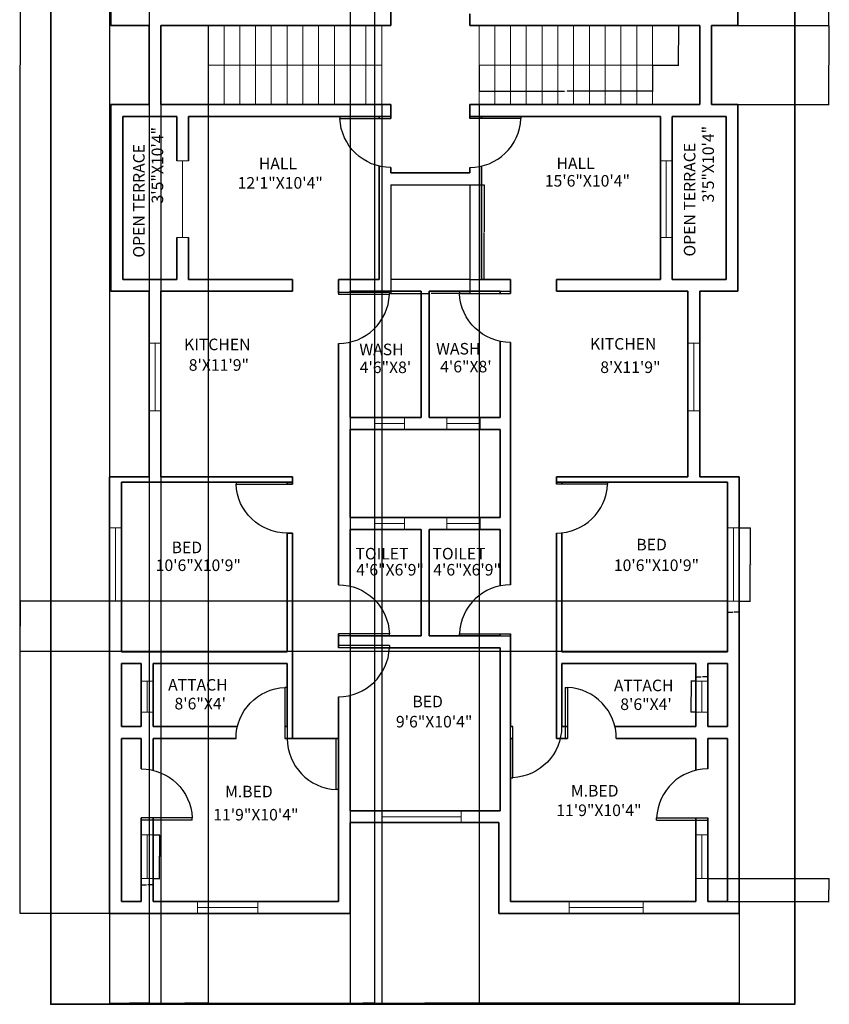
# Model space of a CAD drawing. Units: feet. Extents: x 100807 to 101423, y 154875 to 156331.
# Tile 1 of 8: x 100807 to 101423, y 154875 to 155624. Entities that reach past the tile are written whole.
import ezdxf

# ---------------------------------------------------------------- set-up
doc = ezdxf.new("R2010")
doc.units = ezdxf.units.FT
for name, color, linetype, lineweight in [('A-ANNO-DIMS', 2, 'Continuous', 18), ('A-ANNO-TTLB', 7, 'Continuous', 35), ('A-AREA-IDEN', 7, 'Continuous', 25), ('A-DOOR', 4, 'Continuous', 25), ('A-EQPM-ELEV', 8, 'Continuous', 25), ('A-FLOR-STRS', 3, 'Continuous', 18), ('A-GLAZ', 4, 'Continuous', 18), ('A-WALL', 7, 'Continuous', 35)]:
    doc.layers.add(name, color=color, linetype=linetype, lineweight=lineweight)
doc.styles.get("Standard").update_dxf_attribs({"font": 'arial.ttf'})
doc.dimstyles.get("Standard").update_dxf_attribs({"dimtxt": 0.18, "dimasz": 0.18, "dimexe": 0.18, "dimexo": 0.0625, "dimgap": 0.09, "dimtad": 0, "dimtih": 1, "dimtoh": 1, "dimdec": 4, "dimzin": 0, "dimdsep": 46, "dimtxsty": 'Standard', "dimcen": 0.09, "dimadec": 0, "dimazin": 0, "dimtfac": 1, "dimtdec": 4, "dimtofl": 0, "dimtmove": 0, "dimatfit": 3, "dimfxl": 1, "dimtolj": 1, "dimtzin": 0, "dimarcsym": 0})

# ---------------------------------------------------------------- blocks, each defined once
blk = doc.blocks.new('DR-36')
for p, q in [((0, 36), (0, 0)), ((0, 36), (1.5, 36)), ((1.5, 36), (1.5, 0)), ((0, 0), (1.5, 0))]:
    blk.add_line(p, q)
blk.add_arc((0, 0), 36, 0, 87.61406)
blk = doc.blocks.new('VENT-COURT-A')
for p, q in [((0, 9), (0, 0)), ((22.83, 9), (22.83, 0)), ((22.83, 4.5), (0, 4.5))]:
    blk.add_line(p, q)
blk = doc.blocks.new('WIN-BATH-SIDE')
for p, q in [((0, 23.54), (9, 23.54)), ((4.5, 23.54), (4.5, 0)), ((0, 0), (9, 0))]:
    blk.add_line(p, q)
blk = doc.blocks.new('VENT-COURT-B')
for p, q in [((0, 9), (0, 0)), ((25.42, 9), (25.42, 0)), ((25.42, 4.5), (0, 4.5))]:
    blk.add_line(p, q)
blk = doc.blocks.new('WIN-MBED-SIDE')
for p, q in [((0, 33.08), (9, 33.08)), ((4.5, 33.08), (4.5, 0)), ((0, 0), (9, 0))]:
    blk.add_line(p, q)
blk = doc.blocks.new('WIN-KITCHEN')
for p, q in [((0, 51.58), (9, 51.58)), ((4.5, 51.58), (4.5, 0)), ((0, 0), (9, 0))]:
    blk.add_line(p, q)
blk = doc.blocks.new('WIN-BED-SIDE')
for p, q in [((0, 55.85), (9, 55.85)), ((4.5, 55.85), (4.5, 0)), ((0, 0), (9, 0))]:
    blk.add_line(p, q)
blk = doc.blocks.new('WIN-TERRACE')
for p, q in [((0, 58.29), (9, 58.29)), ((4.5, 58.29), (4.5, 0)), ((0, 0), (9, 0))]:
    blk.add_line(p, q)
blk = doc.blocks.new('WIN-BED-END')
for p, q in [((0, 9), (0, 0)), ((60.14, 9), (60.14, 0)), ((0, 4.5), (60.14, 4.5))]:
    blk.add_line(p, q)
blk = doc.blocks.new('STAIR-FLIGHT-12')
for p, q in [((0, 30), (0, 0)), ((12, 30), (12, 0)), ((24, 30), (24, 0)), ((36, 30), (36, 0)), ((48, 30), (48, 0)), ((60, 30), (60, 0)), ((72, 30), (72, 0)), ((84, 30), (84, 0)), ((96, 30), (96, 0)), ((108, 30), (108, 0)), ((120, 30), (120, 0)), ((132, 30), (132, 0))]:
    blk.add_line(p, q)
blk = doc.blocks.new('LIFT-OUTLINE')
for p, q in [((0, 72), (0, 0)), ((0, 72), (60, 72)), ((60, 72), (60, 0)), ((60, 72), (60, 0)), ((60, 0), (0, 0))]:
    blk.add_line(p, q)
blk = doc.blocks.new('*D18')
at = {"layer": 'A-ANNO-DIMS', "color": 0, "lineweight": -2, "transparency": 16777216}
for p, q in [((101321.09, 155121.03), (101317.44, 155121.03)), ((101317.62, 155120.85), (101317.62, 155109.44)), ((101317.62, 155097.66), (101317.62, 155109.08)), ((101321.09, 155097.48), (101317.44, 155097.48))]:
    blk.add_line(p, q, dxfattribs=at)
at = {"layer": 'A-ANNO-DIMS', "color": 0, "transparency": 16777216}
for points in [[(101317.59, 155120.85), (101317.65, 155120.85), (101317.62, 155121.03)], [(101317.59, 155097.66), (101317.65, 155097.66), (101317.62, 155097.48)]]:
    blk.add_solid(points, dxfattribs=at)
at = {"layer": 'Defpoints', "color": 0, "transparency": 16777216}
for p in [(101321.16, 155121.03), (101317.62, 155097.48), (101321.16, 155097.48)]:
    blk.add_point(p, dxfattribs=at)
at = {"layer": 'A-ANNO-DIMS', "color": 0, "transparency": 16777216, "insert": (101317.62, 155109.26), "char_height": 0.18, "attachment_point": 5}
blk.add_mtext('\\A1;BATH WIN. 24 TYP.', dxfattribs=at)
blk = doc.blocks.new('*D19')
at = {"layer": 'A-ANNO-DIMS', "color": 0, "lineweight": -2, "transparency": 16777216}
for p, q in [((101321.16, 155121.09), (101321.16, 155124.74)), ((101321.34, 155124.56), (101325.2, 155124.56)), ((101329.98, 155124.56), (101326.11, 155124.56)), ((101330.16, 155121.09), (101330.16, 155124.74))]:
    blk.add_line(p, q, dxfattribs=at)
at = {"layer": 'A-ANNO-DIMS', "color": 0, "transparency": 16777216}
for points in [[(101321.34, 155124.59), (101321.34, 155124.53), (101321.16, 155124.56)], [(101329.98, 155124.59), (101329.98, 155124.53), (101330.16, 155124.56)]]:
    blk.add_solid(points, dxfattribs=at)
at = {"layer": 'Defpoints', "color": 0, "transparency": 16777216}
for p in [(101321.16, 155124.56), (101321.16, 155121.03), (101330.16, 155121.03)]:
    blk.add_point(p, dxfattribs=at)
at = {"layer": 'A-ANNO-DIMS', "color": 0, "transparency": 16777216, "insert": (101325.66, 155124.56), "char_height": 0.18, "attachment_point": 5}
blk.add_mtext('\\A1;9 TYP.', dxfattribs=at)
blk = doc.blocks.new('*D20')
at = {"layer": 'A-ANNO-DIMS', "color": 0, "lineweight": -2, "transparency": 16777216}
for p, q in [((100908.22, 155004.3), (100913.3, 155004.3)), ((100913.12, 155004.12), (100913.12, 154987.95)), ((100913.12, 154971.41), (100913.12, 154987.58)), ((100908.22, 154971.23), (100913.3, 154971.23))]:
    blk.add_line(p, q, dxfattribs=at)
at = {"layer": 'A-ANNO-DIMS', "color": 0, "transparency": 16777216}
for points in [[(100913.09, 155004.12), (100913.15, 155004.12), (100913.12, 155004.3)], [(100913.09, 154971.41), (100913.15, 154971.41), (100913.12, 154971.23)]]:
    blk.add_solid(points, dxfattribs=at)
at = {"layer": 'Defpoints', "color": 0, "transparency": 16777216}
for p in [(100908.16, 155004.3), (100908.16, 154971.23), (100913.12, 154971.23)]:
    blk.add_point(p, dxfattribs=at)
at = {"layer": 'A-ANNO-DIMS', "color": 0, "transparency": 16777216, "insert": (100913.12, 154987.76), "char_height": 0.18, "attachment_point": 5}
blk.add_mtext('\\A1;M.BED WIN. 33 TYP.', dxfattribs=at)
blk = doc.blocks.new('*D21')
at = {"layer": 'A-ANNO-DIMS', "color": 0, "lineweight": -2, "transparency": 16777216}
for p, q in [((100899.16, 154971.16), (100899.16, 154966.08)), ((100899.34, 154966.26), (100903.2, 154966.26)), ((100907.98, 154966.26), (100904.11, 154966.26)), ((100908.16, 154971.16), (100908.16, 154966.08))]:
    blk.add_line(p, q, dxfattribs=at)
at = {"layer": 'A-ANNO-DIMS', "color": 0, "transparency": 16777216}
for points in [[(100899.34, 154966.29), (100899.34, 154966.23), (100899.16, 154966.26)], [(100907.98, 154966.29), (100907.98, 154966.23), (100908.16, 154966.26)]]:
    blk.add_solid(points, dxfattribs=at)
at = {"layer": 'Defpoints', "color": 0, "transparency": 16777216}
for p in [(100899.16, 154971.23), (100899.16, 154966.26), (100908.16, 154971.23)]:
    blk.add_point(p, dxfattribs=at)
at = {"layer": 'A-ANNO-DIMS', "color": 0, "transparency": 16777216, "insert": (100903.66, 154966.26), "char_height": 0.18, "attachment_point": 5}
blk.add_mtext('\\A1;9 TYP.', dxfattribs=at)
blk = doc.blocks.new('*D24')
at = {"layer": 'A-ANNO-DIMS', "color": 0, "lineweight": -2, "transparency": 16777216}
for p, q in [((101354.22, 155237.85), (101362.71, 155237.85)), ((101362.53, 155237.67), (101362.53, 155210.11)), ((101362.53, 155182.19), (101362.53, 155209.75)), ((101354.22, 155182.01), (101362.71, 155182.01))]:
    blk.add_line(p, q, dxfattribs=at)
at = {"layer": 'A-ANNO-DIMS', "color": 0, "transparency": 16777216}
for points in [[(101362.5, 155237.67), (101362.56, 155237.67), (101362.53, 155237.85)], [(101362.5, 155182.19), (101362.56, 155182.19), (101362.53, 155182.01)]]:
    blk.add_solid(points, dxfattribs=at)
at = {"layer": 'Defpoints', "color": 0, "transparency": 16777216}
for p in [(101354.16, 155237.85), (101362.53, 155237.85), (101354.16, 155182.01)]:
    blk.add_point(p, dxfattribs=at)
at = {"layer": 'A-ANNO-DIMS', "color": 0, "transparency": 16777216, "insert": (101362.53, 155209.93), "char_height": 0.18, "attachment_point": 5}
blk.add_mtext('\\A1;BED WIN. 56 TYP.', dxfattribs=at)
blk = doc.blocks.new('*D25')
at = {"layer": 'A-ANNO-DIMS', "color": 0, "lineweight": -2, "transparency": 16777216}
for p, q in [((101345.16, 155181.94), (101345.16, 155173.45)), ((101354.16, 155181.94), (101354.16, 155173.45)), ((101345.34, 155173.63), (101349.2, 155173.63)), ((101353.98, 155173.63), (101350.11, 155173.63))]:
    blk.add_line(p, q, dxfattribs=at)
at = {"layer": 'A-ANNO-DIMS', "color": 0, "transparency": 16777216}
for points in [[(101345.34, 155173.66), (101345.34, 155173.6), (101345.16, 155173.63)], [(101353.98, 155173.66), (101353.98, 155173.6), (101354.16, 155173.63)]]:
    blk.add_solid(points, dxfattribs=at)
at = {"layer": 'Defpoints', "color": 0, "transparency": 16777216}
for p in [(101345.16, 155182.01), (101354.16, 155182.01), (101354.16, 155173.63)]:
    blk.add_point(p, dxfattribs=at)
at = {"layer": 'A-ANNO-DIMS', "color": 0, "transparency": 16777216, "insert": (101349.66, 155173.63), "char_height": 0.18, "attachment_point": 5}
blk.add_mtext('\\A1;9 TYP.', dxfattribs=at)
blk = doc.blocks.new('*D30')
at = {"layer": 'A-ANNO-DIMS', "color": 0, "lineweight": -2, "transparency": 16777216}
for p, q in [((101156.16, 155589.49), (101156.16, 155569.58)), ((101288.16, 155589.49), (101288.16, 155569.58)), ((101156.34, 155569.76), (101221.15, 155569.76)), ((101287.98, 155569.76), (101223.16, 155569.76))]:
    blk.add_line(p, q, dxfattribs=at)
at = {"layer": 'A-ANNO-DIMS', "color": 0, "transparency": 16777216}
for points in [[(101156.34, 155569.79), (101156.34, 155569.73), (101156.16, 155569.76)], [(101287.98, 155569.79), (101287.98, 155569.73), (101288.16, 155569.76)]]:
    blk.add_solid(points, dxfattribs=at)
at = {"layer": 'Defpoints', "color": 0, "transparency": 16777216}
for p in [(101156.16, 155589.56), (101288.16, 155589.56), (101288.16, 155569.76)]:
    blk.add_point(p, dxfattribs=at)
at = {"layer": 'A-ANNO-DIMS', "color": 0, "transparency": 16777216, "insert": (101222.16, 155569.76), "char_height": 0.18, "attachment_point": 5}
blk.add_mtext('\\A1;STAIR 132 TYP.', dxfattribs=at)
blk = doc.blocks.new('*D31')
at = {"layer": 'A-ANNO-DIMS', "color": 0, "lineweight": -2, "transparency": 16777216}
for p, q in [((101288.22, 155619.56), (101308.14, 155619.56)), ((101307.96, 155619.38), (101307.96, 155604.74)), ((101307.96, 155589.74), (101307.96, 155604.37)), ((101288.22, 155589.56), (101308.14, 155589.56))]:
    blk.add_line(p, q, dxfattribs=at)
at = {"layer": 'A-ANNO-DIMS', "color": 0, "transparency": 16777216}
for points in [[(101307.93, 155619.38), (101307.99, 155619.38), (101307.96, 155619.56)], [(101307.93, 155589.74), (101307.99, 155589.74), (101307.96, 155589.56)]]:
    blk.add_solid(points, dxfattribs=at)
at = {"layer": 'Defpoints', "color": 0, "transparency": 16777216}
for p in [(101288.16, 155619.56), (101307.96, 155619.56), (101288.16, 155589.56)]:
    blk.add_point(p, dxfattribs=at)
at = {"layer": 'A-ANNO-DIMS', "color": 0, "transparency": 16777216, "insert": (101307.96, 155604.56), "char_height": 0.18, "attachment_point": 5}
blk.add_mtext('\\A1;30 TYP.', dxfattribs=at)
blk = doc.blocks.new('*D32')
at = {"layer": 'A-ANNO-DIMS', "color": 0, "lineweight": -2, "transparency": 16777216}
for p, q in [((101149.22, 155498.58), (101160.14, 155498.58)), ((101159.96, 155498.4), (101159.96, 155462.76)), ((101159.96, 155426.76), (101159.96, 155462.4)), ((101149.22, 155426.58), (101160.14, 155426.58))]:
    blk.add_line(p, q, dxfattribs=at)
at = {"layer": 'A-ANNO-DIMS', "color": 0, "transparency": 16777216}
for points in [[(101159.93, 155498.4), (101159.99, 155498.4), (101159.96, 155498.58)], [(101159.93, 155426.76), (101159.99, 155426.76), (101159.96, 155426.58)]]:
    blk.add_solid(points, dxfattribs=at)
at = {"layer": 'Defpoints', "color": 0, "transparency": 16777216}
for p in [(101149.16, 155498.58), (101159.96, 155498.58), (101149.16, 155426.58)]:
    blk.add_point(p, dxfattribs=at)
at = {"layer": 'A-ANNO-DIMS', "color": 0, "transparency": 16777216, "insert": (101159.96, 155462.58), "char_height": 0.18, "attachment_point": 5}
blk.add_mtext('\\A1;LIFT 72 TYP.', dxfattribs=at)
blk = doc.blocks.new('*D33')
at = {"layer": 'A-ANNO-DIMS', "color": 0, "lineweight": -2, "transparency": 16777216}
for p, q in [((101089.16, 155426.52), (101089.16, 155415.6)), ((101149.16, 155426.52), (101149.16, 155415.6)), ((101089.34, 155415.78), (101118.63, 155415.78)), ((101148.98, 155415.78), (101119.69, 155415.78))]:
    blk.add_line(p, q, dxfattribs=at)
at = {"layer": 'A-ANNO-DIMS', "color": 0, "transparency": 16777216}
for points in [[(101089.34, 155415.81), (101089.34, 155415.75), (101089.16, 155415.78)], [(101148.98, 155415.81), (101148.98, 155415.75), (101149.16, 155415.78)]]:
    blk.add_solid(points, dxfattribs=at)
at = {"layer": 'Defpoints', "color": 0, "transparency": 16777216}
for p in [(101089.16, 155426.58), (101149.16, 155426.58), (101149.16, 155415.78)]:
    blk.add_point(p, dxfattribs=at)
at = {"layer": 'A-ANNO-DIMS', "color": 0, "transparency": 16777216, "insert": (101119.16, 155415.78), "char_height": 0.18, "attachment_point": 5}
blk.add_mtext('\\A1;60 TYP.', dxfattribs=at)
blk = doc.blocks.new('*D34')
at = {"layer": 'A-ANNO-DIMS', "color": 0, "lineweight": -2, "transparency": 16777216}
for p, q in [((100875.16, 154944.52), (100875.16, 154876.25)), ((101354.16, 154944.52), (101354.16, 154876.25)), ((100875.34, 154876.43), (101114.36, 154876.43)), ((101353.98, 154876.43), (101114.95, 154876.43))]:
    blk.add_line(p, q, dxfattribs=at)
at = {"layer": 'A-ANNO-DIMS', "color": 0, "transparency": 16777216}
for points in [[(100875.34, 154876.46), (100875.34, 154876.4), (100875.16, 154876.43)], [(101353.98, 154876.46), (101353.98, 154876.4), (101354.16, 154876.43)]]:
    blk.add_solid(points, dxfattribs=at)
at = {"layer": 'Defpoints', "color": 0, "transparency": 16777216}
for p in [(100875.16, 154944.58), (101354.16, 154944.58), (101354.16, 154876.43)]:
    blk.add_point(p, dxfattribs=at)
at = {"layer": 'A-ANNO-DIMS', "color": 0, "transparency": 16777216, "insert": (101114.66, 154876.43), "char_height": 0.18, "attachment_point": 5}
blk.add_mtext('\\A1;479', dxfattribs=at)
blk = doc.blocks.new('*D35')
at = {"layer": 'A-ANNO-DIMS', "color": 0, "lineweight": -2, "transparency": 16777216}
for p, q in [((100875.09, 156234.58), (100806.83, 156234.58)), ((100807.01, 156234.4), (100807.01, 155589.76)), ((100807.01, 154944.76), (100807.01, 155589.4)), ((100875.09, 154944.58), (100806.83, 154944.58))]:
    blk.add_line(p, q, dxfattribs=at)
at = {"layer": 'A-ANNO-DIMS', "color": 0, "transparency": 16777216}
for points in [[(100806.98, 156234.4), (100807.04, 156234.4), (100807.01, 156234.58)], [(100806.98, 154944.76), (100807.04, 154944.76), (100807.01, 154944.58)]]:
    blk.add_solid(points, dxfattribs=at)
at = {"layer": 'Defpoints', "color": 0, "transparency": 16777216}
for p in [(100807.01, 156234.58), (100875.16, 156234.58), (100875.16, 154944.58)]:
    blk.add_point(p, dxfattribs=at)
at = {"layer": 'A-ANNO-DIMS', "color": 0, "transparency": 16777216, "insert": (100807.01, 155589.58), "char_height": 0.18, "attachment_point": 5}
blk.add_mtext('\\A1;1290', dxfattribs=at)
blk = doc.blocks.new('*D43')
at = {"layer": 'A-ANNO-DIMS', "color": 0, "lineweight": -2, "transparency": 16777216}
for p, q in [((101353.22, 155761.58), (101422.49, 155761.58)), ((101422.31, 155761.4), (101422.31, 155690.75)), ((101422.31, 155619.74), (101422.31, 155690.38)), ((101353.22, 155619.56), (101422.49, 155619.56))]:
    blk.add_line(p, q, dxfattribs=at)
at = {"layer": 'A-ANNO-DIMS', "color": 0, "transparency": 16777216}
for points in [[(101422.28, 155761.4), (101422.34, 155761.4), (101422.31, 155761.58)], [(101422.28, 155619.74), (101422.34, 155619.74), (101422.31, 155619.56)]]:
    blk.add_solid(points, dxfattribs=at)
at = {"layer": 'Defpoints', "color": 0, "transparency": 16777216}
for p in [(101353.16, 155761.58), (101422.31, 155761.58), (101353.16, 155619.56)]:
    blk.add_point(p, dxfattribs=at)
at = {"layer": 'A-ANNO-DIMS', "color": 0, "transparency": 16777216, "insert": (101422.31, 155690.57), "char_height": 0.18, "attachment_point": 5}
blk.add_mtext('\\A1;142.02', dxfattribs=at)
blk = doc.blocks.new('*D44')
at = {"layer": 'A-ANNO-DIMS', "color": 0, "lineweight": -2, "transparency": 16777216}
for p, q in [((101353.22, 155619.56), (101422.49, 155619.56)), ((101422.31, 155619.38), (101422.31, 155589.76)), ((101422.31, 155559.78), (101422.31, 155589.4)), ((101353.22, 155559.6), (101422.49, 155559.6))]:
    blk.add_line(p, q, dxfattribs=at)
at = {"layer": 'A-ANNO-DIMS', "color": 0, "transparency": 16777216}
for points in [[(101422.28, 155619.38), (101422.34, 155619.38), (101422.31, 155619.56)], [(101422.28, 155559.78), (101422.34, 155559.78), (101422.31, 155559.6)]]:
    blk.add_solid(points, dxfattribs=at)
at = {"layer": 'Defpoints', "color": 0, "transparency": 16777216}
for p in [(101353.16, 155619.56), (101422.31, 155619.56), (101353.16, 155559.6)]:
    blk.add_point(p, dxfattribs=at)
at = {"layer": 'A-ANNO-DIMS', "color": 0, "transparency": 16777216, "insert": (101422.31, 155589.58), "char_height": 0.18, "attachment_point": 5}
blk.add_mtext('\\A1;59.96', dxfattribs=at)
blk = doc.blocks.new('*D45')
at = {"layer": 'A-ANNO-DIMS', "color": 0, "lineweight": -2, "transparency": 16777216}
for p, q in [((100875.16, 155902.52), (100875.16, 154876.25)), ((100905.16, 155902.52), (100905.16, 154876.25)), ((100875.34, 154876.43), (100889.94, 154876.43)), ((100904.98, 154876.43), (100890.37, 154876.43))]:
    blk.add_line(p, q, dxfattribs=at)
at = {"layer": 'A-ANNO-DIMS', "color": 0, "transparency": 16777216}
for points in [[(100875.34, 154876.46), (100875.34, 154876.4), (100875.16, 154876.43)], [(100904.98, 154876.46), (100904.98, 154876.4), (100905.16, 154876.43)]]:
    blk.add_solid(points, dxfattribs=at)
at = {"layer": 'Defpoints', "color": 0, "transparency": 16777216}
for p in [(100875.16, 155902.58), (100905.16, 155902.58), (100905.16, 154876.43)]:
    blk.add_point(p, dxfattribs=at)
at = {"layer": 'A-ANNO-DIMS', "color": 0, "transparency": 16777216, "insert": (100890.16, 154876.43), "char_height": 0.18, "attachment_point": 5}
blk.add_mtext('\\A1;30', dxfattribs=at)
blk = doc.blocks.new('*D46')
at = {"layer": 'A-ANNO-DIMS', "color": 0, "lineweight": -2, "transparency": 16777216}
for p, q in [((100914.16, 155619.52), (100914.16, 154876.25)), ((100950.16, 155619.52), (100950.16, 154876.25)), ((100914.34, 154876.43), (100931.94, 154876.43)), ((100949.98, 154876.43), (100932.38, 154876.43))]:
    blk.add_line(p, q, dxfattribs=at)
at = {"layer": 'A-ANNO-DIMS', "color": 0, "transparency": 16777216}
for points in [[(100914.34, 154876.46), (100914.34, 154876.4), (100914.16, 154876.43)], [(100949.98, 154876.46), (100949.98, 154876.4), (100950.16, 154876.43)]]:
    blk.add_solid(points, dxfattribs=at)
at = {"layer": 'Defpoints', "color": 0, "transparency": 16777216}
for p in [(100914.16, 155619.58), (100950.16, 155619.58), (100950.16, 154876.43)]:
    blk.add_point(p, dxfattribs=at)
at = {"layer": 'A-ANNO-DIMS', "color": 0, "transparency": 16777216, "insert": (100932.16, 154876.43), "char_height": 0.18, "attachment_point": 5}
blk.add_mtext('\\A1;36', dxfattribs=at)
blk = doc.blocks.new('*D47')
at = {"layer": 'A-ANNO-DIMS', "color": 0, "lineweight": -2, "transparency": 16777216}
for p, q in [((101082.16, 155559.52), (101082.16, 154876.25)), ((101156.16, 155559.54), (101156.16, 154876.25)), ((101082.34, 154876.43), (101118.94, 154876.43)), ((101155.98, 154876.43), (101119.37, 154876.43))]:
    blk.add_line(p, q, dxfattribs=at)
at = {"layer": 'A-ANNO-DIMS', "color": 0, "transparency": 16777216}
for points in [[(101082.34, 154876.46), (101082.34, 154876.4), (101082.16, 154876.43)], [(101155.98, 154876.46), (101155.98, 154876.4), (101156.16, 154876.43)]]:
    blk.add_solid(points, dxfattribs=at)
at = {"layer": 'Defpoints', "color": 0, "transparency": 16777216}
for p in [(101082.16, 155559.58), (101156.16, 155559.6), (101156.16, 154876.43)]:
    blk.add_point(p, dxfattribs=at)
at = {"layer": 'A-ANNO-DIMS', "color": 0, "transparency": 16777216, "insert": (101119.16, 154876.43), "char_height": 0.18, "attachment_point": 5}
blk.add_mtext('\\A1;74', dxfattribs=at)
blk = doc.blocks.new('*D48')
at = {"layer": 'A-ANNO-DIMS', "color": 0, "lineweight": -2, "transparency": 16777216}
for p, q in [((101058.16, 155933.52), (101058.16, 154876.25)), ((101076.57, 155933.52), (101076.57, 154876.25)), ((101058.34, 154876.43), (101066.99, 154876.43)), ((101076.39, 154876.43), (101067.73, 154876.43))]:
    blk.add_line(p, q, dxfattribs=at)
at = {"layer": 'A-ANNO-DIMS', "color": 0, "transparency": 16777216}
for points in [[(101058.34, 154876.46), (101058.34, 154876.4), (101058.16, 154876.43)], [(101076.39, 154876.46), (101076.39, 154876.4), (101076.57, 154876.43)]]:
    blk.add_solid(points, dxfattribs=at)
at = {"layer": 'Defpoints', "color": 0, "transparency": 16777216}
for p in [(101058.16, 155933.58), (101076.57, 155933.58), (101076.57, 154876.43)]:
    blk.add_point(p, dxfattribs=at)
at = {"layer": 'A-ANNO-DIMS', "color": 0, "transparency": 16777216, "insert": (101067.36, 154876.43), "char_height": 0.18, "attachment_point": 5}
blk.add_mtext('\\A1;18.41', dxfattribs=at)
blk = doc.blocks.new('*D52')
at = {"layer": 'A-ANNO-DIMS', "color": 0, "lineweight": -2, "transparency": 16777216}
for p, q in [((101345.09, 155182.01), (100806.83, 155182.01)), ((100807.01, 155181.83), (100807.01, 155162.97)), ((100807.01, 155143.76), (100807.01, 155162.61)), ((101345.09, 155143.58), (100806.83, 155143.58))]:
    blk.add_line(p, q, dxfattribs=at)
at = {"layer": 'A-ANNO-DIMS', "color": 0, "transparency": 16777216}
for points in [[(100806.98, 155181.83), (100807.04, 155181.83), (100807.01, 155182.01)], [(100806.98, 155143.76), (100807.04, 155143.76), (100807.01, 155143.58)]]:
    blk.add_solid(points, dxfattribs=at)
at = {"layer": 'Defpoints', "color": 0, "transparency": 16777216}
for p in [(101345.16, 155182.01), (100807.01, 155143.58), (101345.16, 155143.58)]:
    blk.add_point(p, dxfattribs=at)
at = {"layer": 'A-ANNO-DIMS', "color": 0, "transparency": 16777216, "insert": (100807.01, 155162.79), "char_height": 0.18, "attachment_point": 5}
blk.add_mtext('\\A1;38.43', dxfattribs=at)
blk = doc.blocks.new('*D54')
at = {"layer": 'A-ANNO-DIMS', "color": 0, "lineweight": -2, "transparency": 16777216}
for p, q in [((101330.22, 154971.23), (101422.49, 154971.23)), ((101422.31, 154971.05), (101422.31, 154962.58)), ((101422.31, 154953.76), (101422.31, 154962.22)), ((101330.22, 154953.58), (101422.49, 154953.58))]:
    blk.add_line(p, q, dxfattribs=at)
at = {"layer": 'A-ANNO-DIMS', "color": 0, "transparency": 16777216}
for points in [[(101422.28, 154971.05), (101422.34, 154971.05), (101422.31, 154971.23)], [(101422.28, 154953.76), (101422.34, 154953.76), (101422.31, 154953.58)]]:
    blk.add_solid(points, dxfattribs=at)
at = {"layer": 'Defpoints', "color": 0, "transparency": 16777216}
for p in [(101330.16, 154971.23), (101422.31, 154971.23), (101330.16, 154953.58)]:
    blk.add_point(p, dxfattribs=at)
at = {"layer": 'A-ANNO-DIMS', "color": 0, "transparency": 16777216, "insert": (101422.31, 154962.4), "char_height": 0.18, "attachment_point": 5}
blk.add_mtext('\\A1;17.647', dxfattribs=at)

msp = doc.modelspace()

# ---------------------------------------------------------------- linework, layer by layer
at = {"layer": 'A-ANNO-TTLB'}
msp.add_lwpolyline([(100830.3877, 156331.4447), (101396.4426, 156331.4447), (101396.4426, 154875.4601), (100830.3877, 154875.4601)], close=True, dxfattribs=at)
at = {"layer": 'A-FLOR-STRS'}
for p, q in [((101082.1564, 155589.5777), (100950.1564, 155589.5777)), ((101082.1564, 155589.5777), (100950.1564, 155589.5777)), ((101082.1564, 155589.5777), (100950.1564, 155589.5777)), ((101082.1564, 155589.5777), (100950.1564, 155589.5777)), ((101156.1564, 155589.5997), (101288.1564, 155589.5997)), ((101156.1564, 155589.5557), (101156.1564, 155589.5997)), ((101156.1564, 155589.5997), (101288.1564, 155589.5997)), ((101156.1564, 155589.5997), (101156.1564, 155589.5557)), ((101156.1564, 155589.5557), (101288.1564, 155589.5557)), ((101156.1564, 155589.5557), (101288.1564, 155589.5557)), ((101168.1564, 155589.5557), (101168.1564, 155589.5997)), ((101168.1564, 155589.5997), (101168.1564, 155589.5557)), ((101180.1564, 155589.5557), (101180.1564, 155589.5997)), ((101180.1564, 155589.5997), (101180.1564, 155589.5557)), ((101192.1564, 155589.5557), (101192.1564, 155589.5997)), ((101192.1564, 155589.5997), (101192.1564, 155589.5557)), ((101204.1564, 155589.5557), (101204.1564, 155589.5997)), ((101204.1564, 155589.5997), (101204.1564, 155589.5557)), ((101216.1564, 155589.5557), (101216.1564, 155589.5997)), ((101216.1564, 155589.5997), (101216.1564, 155589.5557)), ((101228.1564, 155589.5557), (101228.1564, 155589.5997)), ((101228.1564, 155589.5997), (101228.1564, 155589.5557)), ((101240.1564, 155589.5557), (101240.1564, 155589.5997)), ((101240.1564, 155589.5997), (101240.1564, 155589.5557)), ((101252.1564, 155589.5557), (101252.1564, 155589.5997)), ((101252.1564, 155589.5997), (101252.1564, 155589.5557)), ((101264.1564, 155589.5557), (101264.1564, 155589.5997)), ((101264.1564, 155589.5997), (101264.1564, 155589.5557)), ((101276.1564, 155589.5557), (101276.1564, 155589.5997)), ((101276.1564, 155589.5997), (101276.1564, 155589.5557)), ((101288.1564, 155589.5557), (101288.1564, 155589.5997)), ((101288.1564, 155589.5997), (101288.1564, 155589.5557))]:
    msp.add_line(p, q, dxfattribs=at)
at = {"layer": 'A-GLAZ'}
for p, q in [((100942.0387, 154953.5777), (100942.0387, 154944.5777)), ((100942.0387, 154949.0777), (100987.9288, 154949.0777)), ((100987.9288, 154953.5777), (100987.9288, 154944.5777)), ((101224.6478, 154953.5777), (101224.6478, 154944.5777)), ((101224.6478, 154949.0777), (101281.0678, 154949.0777)), ((101281.0678, 154953.5777), (101281.0678, 154944.5777))]:
    msp.add_line(p, q, dxfattribs=at)
at = {"layer": 'A-WALL'}
for p, q in [((100876.1564, 155761.5777), (100876.1564, 155619.5777)), ((101353.1564, 155761.5777), (101353.1564, 155619.5557)), ((101089.1564, 155630.1972), (101089.1564, 155619.5777)), ((101149.1564, 155628.5777), (101149.1564, 155619.5777)), ((100876.1564, 155619.5777), (100905.1564, 155619.5777)), ((100905.1564, 155619.5777), (100876.1564, 155619.5777)), ((100905.1564, 155619.5777), (100905.1564, 155589.5777)), ((101080.1564, 155619.5777), (100914.1564, 155619.5777)), ((100914.1564, 155619.5777), (100914.1564, 155589.5777)), ((100914.1564, 155619.5777), (100926.1564, 155619.5777)), ((101080.1564, 155619.5777), (101089.1564, 155619.5777)), ((101158.1564, 155619.5557), (101149.1564, 155619.5557)), ((101324.1564, 155619.5557), (101153.3986, 155619.5557)), ((101158.1564, 155619.5557), (101324.1564, 155619.5557)), ((101324.1564, 155619.5557), (101312.1564, 155619.5557)), ((101324.1564, 155619.5557), (101324.1564, 155589.5557)), ((101333.1564, 155619.5557), (101333.1564, 155589.5557)), ((101333.1564, 155619.5557), (101353.1564, 155619.5557)), ((100905.1564, 155559.5777), (100905.1564, 155589.5777)), ((100914.1564, 155559.5777), (100914.1564, 155589.5777)), ((101324.1564, 155589.5557), (101324.1564, 155589.5997)), ((101324.1564, 155559.5997), (101324.1564, 155589.5997)), ((101324.1564, 155589.5997), (101324.1564, 155589.5557)), ((101333.1564, 155589.5557), (101333.1564, 155589.5997)), ((101333.1564, 155559.5997), (101333.1564, 155589.5997)), ((101333.1564, 155589.5997), (101333.1564, 155589.5557)), ((100876.1564, 155417.5777), (100876.1564, 155559.5777)), ((100876.1564, 155559.5777), (100905.1564, 155559.5777)), ((100905.1564, 155559.5777), (100876.1564, 155559.5777)), ((100914.1564, 155559.5777), (100926.1564, 155559.5777)), ((101080.1564, 155559.5777), (100914.1564, 155559.5777)), ((101080.1564, 155559.5777), (101089.1564, 155559.5777)), ((101089.1564, 155548.9582), (101089.1564, 155559.5777)), ((101158.1564, 155559.5997), (101149.1564, 155559.5997)), ((101149.1564, 155550.5777), (101149.1564, 155559.5777)), ((101324.1564, 155559.5997), (101153.3986, 155559.5997)), ((101158.1564, 155559.5997), (101324.1564, 155559.5997)), ((101324.1564, 155559.5997), (101312.1564, 155559.5997)), ((101333.1564, 155559.5997), (101353.1564, 155559.5997)), ((101353.1564, 155417.5777), (101353.1564, 155559.5997)), ((100885.1564, 155426.5777), (100885.1564, 155550.5777)), ((100885.1564, 155550.5777), (100926.1564, 155550.5777)), ((100926.1564, 155550.5777), (100926.1564, 155516.8014)), ((100935.1564, 155550.5777), (100935.1564, 155516.8014)), ((101080.1564, 155550.5777), (100935.1564, 155550.5777)), ((101080.1564, 155548.9582), (101080.1564, 155550.5777)), ((101080.1564, 155550.5777), (101089.1564, 155550.5777)), ((101149.1564, 155548.9582), (101149.1564, 155550.5777)), ((101149.1564, 155550.5777), (101294.1564, 155550.5777)), ((101158.1564, 155548.9582), (101158.1564, 155550.5777)), ((101294.1564, 155550.5777), (101294.1564, 155426.5777)), ((101344.1564, 155550.5777), (101303.1564, 155550.5777)), ((101303.1564, 155550.5777), (101303.1564, 155426.5777)), ((101344.1564, 155426.5777), (101344.1564, 155550.5777)), ((101080.1564, 155426.5777), (101080.1564, 155512.7659)), ((101089.1564, 155507.5777), (101089.1564, 155511.7095)), ((101149.1564, 155507.5777), (101149.1564, 155511.7095)), ((101158.1564, 155426.5777), (101158.1564, 155512.7659)), ((101149.1564, 155507.5777), (101089.1564, 155507.5777)), ((100926.1564, 155458.5134), (100926.1564, 155426.5777)), ((100935.1564, 155458.5134), (100935.1564, 155426.5777)), ((100914.1564, 155426.5777), (100885.1564, 155426.5777)), ((100914.1564, 155426.5777), (100926.1564, 155426.5777)), ((100935.1564, 155426.5777), (101014.1564, 155426.5777)), ((101014.1564, 155417.5777), (101014.1564, 155426.5777)), ((101049.1564, 155426.5777), (101080.1564, 155426.5777)), ((101049.1564, 155417.5777), (101049.1564, 155426.5777)), ((101158.1564, 155426.5777), (101180.1564, 155426.5777)), ((101180.1564, 155426.5777), (101158.1564, 155426.5777)), ((101180.1564, 155417.5777), (101180.1564, 155426.5777)), ((101294.1564, 155426.5777), (101215.1564, 155426.5777)), ((101215.1564, 155417.5777), (101215.1564, 155426.5777)), ((101315.1564, 155426.5777), (101303.1564, 155426.5777)), ((101315.1564, 155426.5777), (101344.1564, 155426.5777)), ((100905.1564, 155417.5777), (100876.1564, 155417.5777)), ((100905.1564, 155276.5777), (100905.1564, 155417.5777)), ((100914.1564, 155276.5777), (100914.1564, 155417.5777)), ((100914.1564, 155417.5777), (101010.1564, 155417.5777)), ((100935.1564, 155417.5777), (101014.1564, 155417.5777)), ((101049.1564, 155415.9565), (101049.1564, 155417.5777)), ((101112.1564, 155417.5777), (101058.1564, 155417.5765)), ((101058.1564, 155416.7671), (101058.1564, 155417.5765)), ((101112.1564, 155321.5765), (101112.1564, 155417.5777)), ((101118.1564, 155417.5777), (101161.1564, 155417.5777)), ((101118.1564, 155321.5765), (101118.1564, 155417.5777)), ((101161.1564, 155417.5777), (101172.1564, 155417.5777)), ((101172.1564, 155415.9582), (101172.1564, 155417.5777)), ((101180.1564, 155415.9582), (101180.1564, 155417.5777)), ((101294.1564, 155417.5777), (101215.1564, 155417.5777)), ((101315.1564, 155417.5777), (101219.1564, 155417.5777)), ((101315.1564, 155276.5777), (101315.1564, 155417.5777)), ((101324.1564, 155276.5777), (101324.1564, 155417.5777)), ((101324.1564, 155417.5777), (101353.1564, 155417.5777)), ((101049.1564, 155194.4447), (101049.1564, 155377.8989)), ((101058.1564, 155321.5765), (101058.1564, 155378.9552)), ((101172.1564, 155321.5765), (101172.1564, 155379.5417)), ((101180.1564, 155194.4447), (101180.1564, 155378.7095)), ((101058.1564, 155321.5765), (101112.1564, 155321.5765)), ((101118.1564, 155321.5765), (101172.1564, 155321.5765)), ((101058.1564, 155312.5765), (101172.1564, 155312.5765)), ((101058.1564, 155245.5765), (101058.1564, 155312.5765)), ((101172.1564, 155245.5765), (101172.1564, 155312.5765)), ((100875.1564, 155143.5777), (100875.1564, 155276.5777)), ((100905.1564, 155276.5777), (100875.1564, 155276.5777)), ((100884.1564, 155143.5777), (100884.1564, 155272.5777)), ((100884.1564, 155272.5777), (101014.1564, 155272.5777)), ((100914.1564, 155276.5777), (101010.1564, 155276.5777)), ((101010.1564, 155276.5777), (101014.1564, 155276.5777)), ((101010.1564, 155272.5777), (101010.1564, 155270.9582)), ((101010.1564, 155270.9582), (101014.1564, 155270.9582)), ((101014.1564, 155276.5777), (101014.1564, 155270.9582)), ((101215.1564, 155276.5777), (101215.1564, 155270.9582)), ((101219.1564, 155276.5777), (101215.1564, 155276.5777)), ((101345.1564, 155272.5777), (101215.1564, 155272.5777)), ((101315.1564, 155276.5777), (101219.1564, 155276.5777)), ((101219.1564, 155272.5777), (101219.1564, 155270.9582)), ((101324.1564, 155276.5777), (101354.1564, 155276.5777)), ((101345.1564, 155143.5777), (101345.1564, 155272.5777)), ((101354.1564, 155143.5777), (101354.1564, 155276.5777)), ((101172.1564, 155245.5765), (101058.1564, 155245.5765)), ((101172.1564, 155245.5765), (101118.1564, 155245.5765)), ((101010.1564, 155233.7095), (101014.1564, 155233.7281)), ((101010.1564, 155233.7095), (101010.1564, 155143.5777)), ((101014.1564, 155233.7281), (101014.1564, 155077.5777)), ((101112.1564, 155236.5765), (101058.1564, 155236.5765)), ((101058.1564, 155193.3884), (101058.1564, 155236.5765)), ((101112.1564, 155155.5765), (101112.1564, 155236.5765)), ((101172.1564, 155236.5765), (101118.1564, 155236.5765)), ((101118.1564, 155155.5765), (101118.1564, 155236.5765)), ((101172.1564, 155193.6125), (101172.1564, 155236.5765)), ((101215.1564, 155233.7095), (101215.1564, 155086.5777)), ((101219.1564, 155233.9159), (101219.1564, 155143.5777)), ((101049.1564, 155146.5765), (101049.1564, 155157.196)), ((101058.1564, 155155.5765), (101058.1564, 155157.196)), ((101112.1564, 155155.5765), (101058.1564, 155155.5765)), ((101172.1564, 155155.5765), (101118.1564, 155155.5765)), ((101172.1564, 155155.5765), (101172.1564, 155157.196)), ((101180.1564, 155086.5777), (101180.1564, 155157.196)), ((100875.1564, 155143.5777), (100875.1564, 154944.5777)), ((101010.1564, 155143.5777), (100884.1564, 155143.5777)), ((101172.1564, 155146.5765), (101058.1564, 155146.5765)), ((101172.1564, 155022.5765), (101172.1564, 155146.5765)), ((101219.1564, 155143.5777), (101345.1564, 155143.5777)), ((101354.1564, 155143.5777), (101354.1564, 154944.5777)), ((100884.1564, 155134.5777), (100899.1564, 155134.5777)), ((100884.1564, 155134.5777), (100884.1564, 155086.5777)), ((100899.1564, 155086.5777), (100899.1564, 155134.5777)), ((100908.1564, 155086.5777), (100908.1564, 155134.5777)), ((100908.1564, 155134.5777), (101010.1564, 155134.5777)), ((101010.1564, 155134.5777), (101010.1564, 155086.5777)), ((101014.1564, 155134.5777), (101014.1564, 155086.5777)), ((101215.1564, 155134.5777), (101215.1564, 155086.5777)), ((101321.1564, 155134.5777), (101219.1564, 155134.5777)), ((101219.1564, 155134.5777), (101219.1564, 155086.5777)), ((101321.1564, 155086.5777), (101321.1564, 155134.5777)), ((101330.1564, 155086.5777), (101330.1564, 155134.5777)), ((101345.1564, 155134.5777), (101330.1564, 155134.5777)), ((101345.1564, 155134.5777), (101345.1564, 155086.5777)), ((101049.1564, 155077.5777), (101049.1564, 155109.3278)), ((101058.1564, 155022.5765), (101058.1564, 155110.3842)), ((100899.1564, 155086.5777), (100884.1564, 155086.5777)), ((100972.3446, 155086.5777), (100908.1564, 155086.5777)), ((101010.1564, 155086.5777), (101008.5369, 155086.5777)), ((101180.1564, 155086.5777), (101181.7759, 155086.5777)), ((101215.1564, 155086.5777), (101215.1564, 155077.5777)), ((101219.1564, 155086.5777), (101223.3792, 155086.5777)), ((101259.5661, 155086.5777), (101321.1564, 155086.5777)), ((101330.1564, 155086.5777), (101345.1564, 155086.5777)), ((100899.1564, 155077.5777), (100884.1564, 155077.5777)), ((100884.1564, 155077.5777), (100884.1564, 154953.5777)), ((100899.1564, 155077.5777), (100899.1564, 155054.4459)), ((100971.2882, 155077.5777), (100908.1564, 155077.5777)), ((100908.1564, 155077.5777), (100908.1564, 155053.3896)), ((101049.1564, 155077.5777), (101008.5369, 155077.5777)), ((101049.1564, 154953.5777), (101049.1564, 155077.5777)), ((101180.1564, 154953.5777), (101180.1564, 155077.5777)), ((101180.1564, 155077.5777), (101181.7759, 155077.5777)), ((101215.1564, 155077.5777), (101223.3792, 155077.5777)), ((101260.6279, 155077.5777), (101321.1564, 155077.5777)), ((101321.1564, 155077.5777), (101321.1564, 155053.3896)), ((101330.1564, 155077.5777), (101345.1564, 155077.5777)), ((101330.1564, 155077.5777), (101330.1564, 155054.4459)), ((101345.1564, 155077.5777), (101345.1564, 154953.5777)), ((100899.1564, 155017.1972), (100899.1564, 154953.5777)), ((100908.1564, 155017.1972), (100908.1564, 154953.5777)), ((101058.1564, 155022.5765), (101172.1564, 155022.5765)), ((101321.1564, 155017.1972), (101321.1564, 154953.5777)), ((101330.1564, 155017.1972), (101330.1564, 154953.5777)), ((101058.1564, 155013.5765), (101171.1564, 155013.5765)), ((101058.1564, 154944.5777), (101058.1564, 155013.5765)), ((101171.1564, 154944.5777), (101171.1564, 155013.5765)), ((101058.1564, 154944.5777), (101058.1564, 154968.5777)), ((101058.1564, 154944.5777), (101058.1564, 154968.5777)), ((101171.1564, 154944.5777), (101171.1564, 154968.5777)), ((101058.1564, 154944.5777), (101058.1564, 154956.5777)), ((101171.1564, 154944.5777), (101171.1564, 154956.5777)), ((100884.1564, 154953.5777), (100899.1564, 154953.5777)), ((100908.1564, 154953.5777), (101049.1564, 154953.5777)), ((101321.1564, 154953.5777), (101180.1564, 154953.5777)), ((101345.1564, 154953.5777), (101330.1564, 154953.5777)), ((100875.1564, 154944.5777), (101058.1564, 154944.5777)), ((101354.1564, 154944.5777), (101171.1564, 154944.5777))]:
    msp.add_line(p, q, dxfattribs=at)

# ---------------------------------------------------------------- block references
at = {"layer": 'A-DOOR', "yscale": 1.079672442471032, "zscale": 1.079672442471032}
for p, xscale, rotation in [((101089.1564, 155550.5777), -1.079672442471032, 90), ((101149.1564, 155550.5777), 1.079672442471032, 269.9999999999631), ((101049.1564, 155416.7671), 1.079672442471032, 269.9999999999631), ((101180.1564, 155417.5777), -1.079672442471032, 90), ((101010.1564, 155272.5777), -1.079672442471032, 90), ((101215.1564, 155272.5777), 1.079672442471032, 269.9999999999631), ((101049.1564, 155155.5765), -1.079672442471032, 270.0000000000369), ((101180.1564, 155155.5765), 1.079672442471032, 90.00000000000003), ((101049.1564, 155148.196), 1.079672442471032, 269.9999999999631), ((101180.1564, 155086.5777), -1.079672442471032, 180), ((101049.1564, 155077.5777), 1.079672442471032, 180), ((100899.1564, 155015.5777), -1.079672442471032, 270.0000000000369), ((101330.1564, 155015.5777), 1.079672442471032, 90.00000000000003)]:
    msp.add_blockref('DR-36', p, dxfattribs=dict(at, xscale=xscale, rotation=rotation))
for p, xscale in [((101010.1564, 155077.5777), -1.079672442471032), ((101221.7597, 155077.5548), 1.079672442471032)]:
    msp.add_blockref('DR-36', p, dxfattribs=dict(at, xscale=xscale))
at = {"layer": 'A-EQPM-ELEV'}
msp.add_blockref('LIFT-OUTLINE', (101089.1564, 155426.5777), dxfattribs=at)
at = {"layer": 'A-FLOR-STRS'}
for p in [(100950.1564, 155589.5777), (101156.1564, 155589.5557), (101156.1564, 155559.5997)]:
    msp.add_blockref('STAIR-FLIGHT-12', p, dxfattribs=at)
at = {"layer": 'A-FLOR-STRS', "rotation": 180}
msp.add_blockref('STAIR-FLIGHT-12', (101082.1564, 155589.5777), dxfattribs=at)
at = {"layer": 'A-GLAZ', "rotation": 180}
for name, p in [('WIN-TERRACE', (100935.1564, 155516.8014)), ('WIN-KITCHEN', (100914.1564, 155378.2313)), ('WIN-KITCHEN', (101324.1564, 155378.2313)), ('VENT-COURT-A', (101099.3962, 155321.5765)), ('VENT-COURT-B', (101157.0816, 155245.5765)), ('WIN-BATH-SIDE', (100908.1564, 155121.0279)), ('WIN-BATH-SIDE', (101330.1564, 155121.0279)), ('WIN-MBED-SIDE', (100908.1564, 155004.3014))]:
    msp.add_blockref(name, p, dxfattribs=at)
at = {"layer": 'A-GLAZ'}
for name, p in [('WIN-TERRACE', (101294.1564, 155458.5134)), ('VENT-COURT-B', (101131.6622, 155312.5765)), ('VENT-COURT-A', (101076.5662, 155236.5765)), ('WIN-BED-SIDE', (100875.1564, 155182.0053)), ('WIN-BED-SIDE', (101345.1564, 155182.0053)), ('WIN-BED-END', (101082.3615, 155013.5765)), ('WIN-MBED-SIDE', (101321.1564, 154971.2251))]:
    msp.add_blockref(name, p, dxfattribs=at)

# ---------------------------------------------------------------- texts
at = {"layer": 'A-ANNO-DIMS'}
for p in [(100915.8734, 155484.3201), (101334.9102, 155485.1377)]:
    msp.add_text('3\'5"X10\'4"', height=8.78822, rotation=90, dxfattribs=at).set_placement(p)
for s, height, p in [('12\'1"X10\'4"', 8.788223, (100972.5123, 155495.6021)), ('15\'6"X10\'4"', 8.788223, (101206.2046, 155497.1804)), ('8\'X11\'9"', 8.78822, (100935.3222, 155357.1529)), ('4\'6"X8\'', 8.78822, (101065.3908, 155355.369)), ('4\'6"X8\'', 8.78822, (101126.6018, 155355.9103)), ('8\'X11\'9"', 8.78822, (101248.4226, 155355.4527)), ('10\'6"X10\'9"', 8.788223, (100910.1724, 155204.8929)), ('10\'6"X10\'9"', 8.788223, (101258.7501, 155204.8929)), ('4\'6"X6\'9"', 8.78822, (101062.7368, 155201.4674)), ('4\'6"X6\'9"', 8.78822, (101121.3373, 155201.4674)), ('8\'6"X4\'', 8.78822, (100924.4842, 155099.6741)), ('8\'6"X4\'', 8.78822, (101263.6348, 155099.2265)), ('9\'6"X10\'4"', 8.78822, (101092.9589, 155085.9526)), ('11\'9"X10\'4"', 8.788223, (100953.9752, 155015.2176)), ('11\'9"X10\'4"', 8.788223, (101214.976, 155018.5993))]:
    msp.add_text(s, height=height, dxfattribs=at).set_placement(p)
at = {"layer": 'A-AREA-IDEN'}
for p in [(100901.7559, 155443.1905), (101320.7927, 155444.0081)]:
    msp.add_text('OPEN TERRACE', height=8.788223, rotation=90, dxfattribs=at).set_placement(p)
for s, p in [('HALL', (100988.6403, 155510.2673)), ('HALL', (101215.1022, 155510.51)), ('KITCHEN', (100931.7636, 155372.7921)), ('WASH', (101065.1121, 155368.9715)), ('WASH', (101123.5377, 155369.5127)), ('KITCHEN', (101240.5933, 155373.2255)), ('BED', (100922.2934, 155218.4471)), ('BED', (101275.8625, 155220.5846)), ('TOILET', (101062.1786, 155213.7185)), ('TOILET', (101120.779, 155213.7185)), ('ATTACH', (100919.6163, 155113.9684)), ('ATTACH', (101258.7669, 155113.5208)), ('BED', (101105.5032, 155101.267)), ('M.BED', (100962.9517, 155032.8262)), ('M.BED', (101226.0509, 155033.4045))]:
    msp.add_text(s, height=8.78822, dxfattribs=at).set_placement(p)

# ---------------------------------------------------------------- dimensions: what is measured, and where the dimension line sits
at = {"layer": 'A-ANNO-DIMS'}
for base, p1, p2, override, picture, middle in [((100807.0064, 156234.5777), (100875.1564, 154944.5777), (100875.1564, 156234.5777), {"dimdec": 0, "dimlfac": 1, "dimrnd": 0, "dimzin": 0, "dimdsep": 46, "dimlunit": 2}, '*D35', (100807.0064, 155589.5777)), ((101422.3064, 155761.5777), (101353.1564, 155619.5557), (101353.1564, 155761.5777), {"dimdec": 2, "dimlfac": 1, "dimrnd": 0, "dimzin": 0, "dimdsep": 46, "dimlunit": 2}, '*D43', (101422.3064, 155690.5667)), ((101422.3064, 155619.5557), (101353.1564, 155559.5997), (101353.1564, 155619.5557), {"dimdec": 2, "dimlfac": 1, "dimrnd": 0, "dimzin": 0, "dimdsep": 46, "dimlunit": 2}, '*D44', (101422.3064, 155589.5777)), ((100807.0064, 155143.5777), (101345.1564, 155182.0053), (101345.1564, 155143.5777), {"dimdec": 2, "dimlfac": 1, "dimrnd": 0, "dimzin": 0, "dimdsep": 46, "dimlunit": 2}, '*D52', (100807.0064, 155162.7915)), ((101422.3064, 154971.2251), (101330.1564, 154953.5777), (101330.1564, 154971.2251), {"dimdec": 3, "dimlfac": 1, "dimrnd": 0, "dimzin": 0, "dimdsep": 46, "dimlunit": 2}, '*D54', (101422.3064, 154962.4014))]:
    dim = msp.add_linear_dim(base=base, p1=p1, p2=p2, angle=90, dimstyle='Standard', override=override, dxfattribs=at)
    dim.commit()
    dim.dimension.update_dxf_attribs({"geometry": picture, "text_midpoint": middle})
for base, p1, p2, override, picture, middle in [((101076.5662, 154876.4277), (101058.1564, 155933.5789), (101076.5662, 155933.5789), {"dimdec": 2, "dimlfac": 1, "dimrnd": 0, "dimzin": 0, "dimdsep": 46, "dimlunit": 2}, '*D48', (101067.3613, 154876.4277)), ((100905.1564, 154876.4277), (100875.1564, 155902.5777), (100905.1564, 155902.5777), {"dimdec": 0, "dimlfac": 1, "dimrnd": 0, "dimzin": 0, "dimdsep": 46, "dimlunit": 2}, '*D45', (100890.1564, 154876.4277)), ((100950.1564, 154876.4277), (100914.1564, 155619.5777), (100950.1564, 155619.5777), {"dimdec": 0, "dimlfac": 1, "dimrnd": 0, "dimzin": 0, "dimdsep": 46, "dimlunit": 2}, '*D46', (100932.1564, 154876.4277)), ((101156.1564, 154876.4277), (101082.1564, 155559.5777), (101156.1564, 155559.5997), {"dimdec": 0, "dimlfac": 1, "dimrnd": 0, "dimzin": 0, "dimdsep": 46, "dimlunit": 2}, '*D47', (101119.1564, 154876.4277)), ((101354.1564, 154876.4277), (100875.1564, 154944.5777), (101354.1564, 154944.5777), {"dimdec": 0, "dimlfac": 1, "dimrnd": 0, "dimzin": 0, "dimdsep": 46, "dimlunit": 2}, '*D34', (101114.6564, 154876.4277))]:
    dim = msp.add_linear_dim(base=base, p1=p1, p2=p2, dimstyle='Standard', override=override, dxfattribs=at)
    dim.commit()
    dim.dimension.update_dxf_attribs({"geometry": picture, "text_midpoint": middle})
for base, p1, p2, angle, text, picture, middle in [((101307.9564, 155619.5557), (101288.1564, 155589.5557), (101288.1564, 155619.5557), 90, '<> TYP.', '*D31', (101307.9564, 155604.5557)), ((101159.9564, 155498.5777), (101149.1564, 155426.5777), (101149.1564, 155498.5777), 90, 'LIFT <> TYP.', '*D32', (101159.9564, 155462.5777)), ((101362.5335, 155237.8525), (101354.1564, 155182.0053), (101354.1564, 155237.8525), 90, 'BED WIN. <> TYP.', '*D24', (101362.5335, 155209.9289)), ((101321.1564, 155124.5593), (101330.1564, 155121.0279), (101321.1564, 155121.0279), 180, '<> TYP.', '*D19', (101325.6564, 155124.5593)), ((101317.625, 155097.4849), (101321.1564, 155121.0279), (101321.1564, 155097.4849), 270, 'BATH WIN. <> TYP.', '*D18', (101317.625, 155109.2564)), ((100913.1179, 154971.2251), (100908.1564, 155004.3014), (100908.1564, 154971.2251), 270, 'M.BED WIN. <> TYP.', '*D20', (100913.1179, 154987.7632)), ((100899.1564, 154966.2636), (100908.1564, 154971.2251), (100899.1564, 154971.2251), 180, '<> TYP.', '*D21', (100903.6564, 154966.2636))]:
    dim = msp.add_linear_dim(base=base, p1=p1, p2=p2, angle=angle, text=text, dimstyle='Standard', override={"dimdec": 0, "dimlfac": 1, "dimrnd": 0, "dimzin": 0, "dimdsep": 46, "dimlunit": 2}, dxfattribs=at)
    dim.commit()
    dim.dimension.update_dxf_attribs({"geometry": picture, "text_midpoint": middle})
for base, p1, p2, text, picture, middle in [((101288.1564, 155569.7557), (101156.1564, 155589.5557), (101288.1564, 155589.5557), 'STAIR <> TYP.', '*D30', (101222.1564, 155569.7557)), ((101149.1564, 155415.7777), (101089.1564, 155426.5777), (101149.1564, 155426.5777), '<> TYP.', '*D33', (101119.1564, 155415.7777)), ((101354.1564, 155173.6283), (101345.1564, 155182.0053), (101354.1564, 155182.0053), '<> TYP.', '*D25', (101349.6564, 155173.6283))]:
    dim = msp.add_linear_dim(base=base, p1=p1, p2=p2, text=text, dimstyle='Standard', override={"dimdec": 0, "dimlfac": 1, "dimrnd": 0, "dimzin": 0, "dimdsep": 46, "dimlunit": 2}, dxfattribs=at)
    dim.commit()
    dim.dimension.update_dxf_attribs({"geometry": picture, "text_midpoint": middle})

doc.saveas('drawing.dxf')
